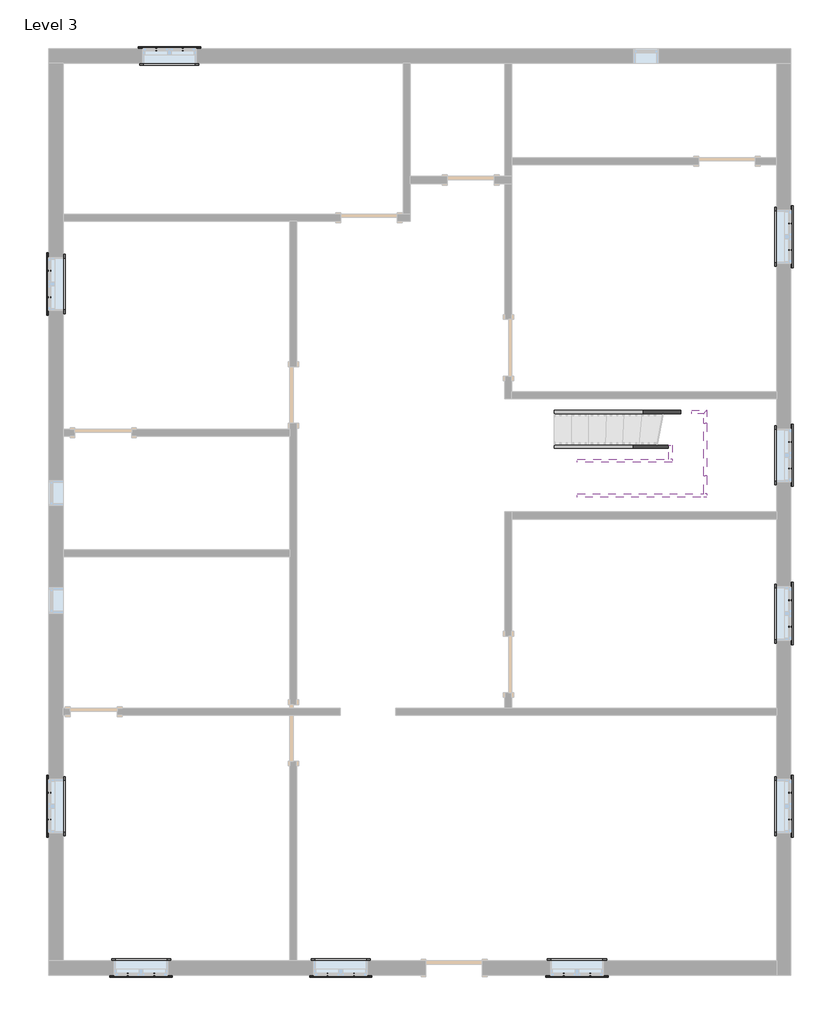
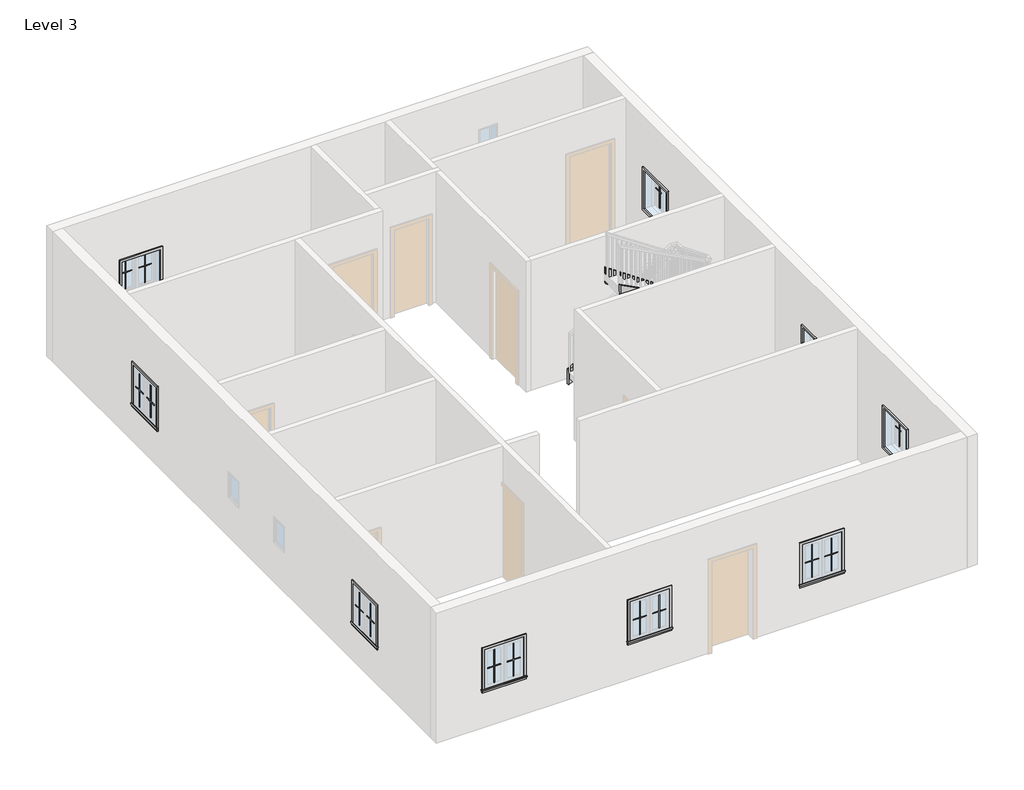
# One storey, part 3 of 3: 40 proxies, 9 members.
"""IFC4 building model written with IfcOpenShell, lengths in millimetres."""

from ifc_helpers import new_model, si_unit, frame, origin, place, context, project, spatial, polyline, outline, extrude, transform, mapped, element, save
from components import muntin_pattern_2x2_muntin_pattern_2x2_b3fe6957, muntin_pattern_2x2_muntin_pattern_2x2_3e0ecaf2, trim_window_exterior_flat_with_sill_41619996, trim_window_interior_flat_picture_frame_51c85655

model = new_model("IFC4")

# Units and contexts
model_context = context("Model", 3, world=origin())
ifc_project = project(units=[si_unit("LENGTHUNIT", "METRE", prefix="MILLI")], contexts=[model_context])

# Site, building, storey
site = spatial("IfcSite", under=ifc_project)
building = spatial("IfcBuilding", under=site)
storey = spatial("IfcBuildingStorey", under=building, Name="Level 3", Elevation=3200.4)

# Proxies
placement = place(None, origin())
muntin_pattern_2x2_muntin_pattern_2x2_shape = muntin_pattern_2x2_muntin_pattern_2x2_b3fe6957(model_context)
element("IfcBuildingElementProxy", 1, Name="Muntin Pattern_2x2 : Muntin Pattern_2x2", ObjectType="Muntin Pattern_2x2 : Muntin Pattern_2x2", at=placement, inside=storey, context=model_context, shape_type="MappedRepresentation", body=[
    mapped(muntin_pattern_2x2_muntin_pattern_2x2_shape, transform((-5581.2368007, 9072.452558, 4184.65), x_axis=(1.0, 0.0, 0.0), y_axis=(0.0, 1.0, 0.0), z_axis=(0.0, 0.0, 1.0))),
])
element("IfcBuildingElementProxy", 2, Name="Muntin Pattern_2x2 : Muntin Pattern_2x2", ObjectType="Muntin Pattern_2x2 : Muntin Pattern_2x2", at=placement, inside=storey, context=model_context, shape_type="MappedRepresentation", body=[
    mapped(muntin_pattern_2x2_muntin_pattern_2x2_shape, transform((-7300.4993007, 5076.715058, 4184.65), x_axis=(0.0, 1.0, 0.0), y_axis=(-1.0, 0.0, 0.0), z_axis=(0.0, 0.0, 1.0))),
])
element("IfcBuildingElementProxy", 3, Name="Muntin Pattern_2x2 : Muntin Pattern_2x2", ObjectType="Muntin Pattern_2x2 : Muntin Pattern_2x2", at=placement, inside=storey, context=model_context, shape_type="MappedRepresentation", body=[
    mapped(muntin_pattern_2x2_muntin_pattern_2x2_shape, transform((4643.8506993, 6267.340058, 4184.65), x_axis=(0.0, -1.0, 0.0), y_axis=(1.0, 0.0, 0.0), z_axis=(0.0, 0.0, 1.0))),
])
element("IfcBuildingElementProxy", 4, Name="Muntin Pattern_2x2 : Muntin Pattern_2x2", ObjectType="Muntin Pattern_2x2 : Muntin Pattern_2x2", at=placement, inside=storey, context=model_context, shape_type="MappedRepresentation", body=[
    mapped(muntin_pattern_2x2_muntin_pattern_2x2_shape, transform((4643.8506993, 2743.090058, 4184.65), x_axis=(0.0, -1.0, 0.0), y_axis=(1.0, 0.0, 0.0), z_axis=(0.0, 0.0, 1.0))),
])
element("IfcBuildingElementProxy", 5, Name="Muntin Pattern_2x2 : Muntin Pattern_2x2", ObjectType="Muntin Pattern_2x2 : Muntin Pattern_2x2", at=placement, inside=storey, context=model_context, shape_type="MappedRepresentation", body=[
    mapped(muntin_pattern_2x2_muntin_pattern_2x2_shape, transform((4643.8506993, 190.390058, 4184.65), x_axis=(0.0, -1.0, 0.0), y_axis=(1.0, 0.0, 0.0), z_axis=(0.0, 0.0, 1.0))),
])
element("IfcBuildingElementProxy", 6, Name="Muntin Pattern_2x2 : Muntin Pattern_2x2", ObjectType="Muntin Pattern_2x2 : Muntin Pattern_2x2", at=placement, inside=storey, context=model_context, shape_type="MappedRepresentation", body=[
    mapped(muntin_pattern_2x2_muntin_pattern_2x2_shape, transform((4643.8506993, -2914.759942, 4184.65), x_axis=(0.0, -1.0, 0.0), y_axis=(1.0, 0.0, 0.0), z_axis=(0.0, 0.0, 1.0))),
])
element("IfcBuildingElementProxy", 7, Name="Muntin Pattern_2x2 : Muntin Pattern_2x2", ObjectType="Muntin Pattern_2x2 : Muntin Pattern_2x2", at=placement, inside=storey, context=model_context, shape_type="MappedRepresentation", body=[
    mapped(muntin_pattern_2x2_muntin_pattern_2x2_shape, transform((1419.6381993, -5843.697442, 4184.65), x_axis=(-1.0, 0.0, 0.0), y_axis=(0.0, -1.0, 0.0), z_axis=(0.0, 0.0, 1.0))),
])
element("IfcBuildingElementProxy", 8, Name="Muntin Pattern_2x2 : Muntin Pattern_2x2", ObjectType="Muntin Pattern_2x2 : Muntin Pattern_2x2", at=placement, inside=storey, context=model_context, shape_type="MappedRepresentation", body=[
    mapped(muntin_pattern_2x2_muntin_pattern_2x2_shape, transform((-2390.3618007, -5843.697442, 4184.65), x_axis=(-1.0, 0.0, 0.0), y_axis=(0.0, -1.0, 0.0), z_axis=(0.0, 0.0, 1.0))),
])
element("IfcBuildingElementProxy", 9, Name="Muntin Pattern_2x2 : Muntin Pattern_2x2", ObjectType="Muntin Pattern_2x2 : Muntin Pattern_2x2", at=placement, inside=storey, context=model_context, shape_type="MappedRepresentation", body=[
    mapped(muntin_pattern_2x2_muntin_pattern_2x2_shape, transform((-5609.8118007, -5843.697442, 4184.65), x_axis=(-1.0, 0.0, 0.0), y_axis=(0.0, -1.0, 0.0), z_axis=(0.0, 0.0, 1.0))),
])
element("IfcBuildingElementProxy", 10, Name="Muntin Pattern_2x2 : Muntin Pattern_2x2", ObjectType="Muntin Pattern_2x2 : Muntin Pattern_2x2", at=placement, inside=storey, context=model_context, shape_type="MappedRepresentation", body=[
    mapped(muntin_pattern_2x2_muntin_pattern_2x2_shape, transform((-7300.4993007, -3343.384942, 4184.65), x_axis=(0.0, 1.0, 0.0), y_axis=(-1.0, 0.0, 0.0), z_axis=(0.0, 0.0, 1.0))),
])
muntin_pattern_2x2_muntin_pattern_2x2_2_shape = muntin_pattern_2x2_muntin_pattern_2x2_3e0ecaf2(model_context)
element("IfcBuildingElementProxy", 11, Name="Muntin Pattern_2x2 : Muntin Pattern_2x2", ObjectType="Muntin Pattern_2x2 : Muntin Pattern_2x2", at=placement, inside=storey, context=model_context, shape_type="MappedRepresentation", body=[
    mapped(muntin_pattern_2x2_muntin_pattern_2x2_2_shape, transform((-5152.6118007, 9072.452558, 4184.65), x_axis=(-1.0, 0.0, 0.0), y_axis=(0.0, -1.0, 0.0), z_axis=(0.0, 0.0, 1.0))),
])
element("IfcBuildingElementProxy", 12, Name="Muntin Pattern_2x2 : Muntin Pattern_2x2", ObjectType="Muntin Pattern_2x2 : Muntin Pattern_2x2", at=placement, inside=storey, context=model_context, shape_type="MappedRepresentation", body=[
    mapped(muntin_pattern_2x2_muntin_pattern_2x2_2_shape, transform((-7300.4993007, 5505.340058, 4184.65), x_axis=(0.0, -1.0, 0.0), y_axis=(1.0, 0.0, 0.0), z_axis=(0.0, 0.0, 1.0))),
])
element("IfcBuildingElementProxy", 13, Name="Muntin Pattern_2x2 : Muntin Pattern_2x2", ObjectType="Muntin Pattern_2x2 : Muntin Pattern_2x2", at=placement, inside=storey, context=model_context, shape_type="MappedRepresentation", body=[
    mapped(muntin_pattern_2x2_muntin_pattern_2x2_2_shape, transform((4643.8506993, 5838.715058, 4184.65), x_axis=(0.0, 1.0, 0.0), y_axis=(-1.0, 0.0, 0.0), z_axis=(0.0, 0.0, 1.0))),
])
element("IfcBuildingElementProxy", 14, Name="Muntin Pattern_2x2 : Muntin Pattern_2x2", ObjectType="Muntin Pattern_2x2 : Muntin Pattern_2x2", at=placement, inside=storey, context=model_context, shape_type="MappedRepresentation", body=[
    mapped(muntin_pattern_2x2_muntin_pattern_2x2_2_shape, transform((4643.8506993, 2314.465058, 4184.65), x_axis=(0.0, 1.0, 0.0), y_axis=(-1.0, 0.0, 0.0), z_axis=(0.0, 0.0, 1.0))),
])
element("IfcBuildingElementProxy", 15, Name="Muntin Pattern_2x2 : Muntin Pattern_2x2", ObjectType="Muntin Pattern_2x2 : Muntin Pattern_2x2", at=placement, inside=storey, context=model_context, shape_type="MappedRepresentation", body=[
    mapped(muntin_pattern_2x2_muntin_pattern_2x2_2_shape, transform((4643.8506993, -238.234942, 4184.65), x_axis=(0.0, 1.0, 0.0), y_axis=(-1.0, 0.0, 0.0), z_axis=(0.0, 0.0, 1.0))),
])
element("IfcBuildingElementProxy", 16, Name="Muntin Pattern_2x2 : Muntin Pattern_2x2", ObjectType="Muntin Pattern_2x2 : Muntin Pattern_2x2", at=placement, inside=storey, context=model_context, shape_type="MappedRepresentation", body=[
    mapped(muntin_pattern_2x2_muntin_pattern_2x2_2_shape, transform((4643.8506993, -3343.384942, 4184.65), x_axis=(0.0, 1.0, 0.0), y_axis=(-1.0, 0.0, 0.0), z_axis=(0.0, 0.0, 1.0))),
])
element("IfcBuildingElementProxy", 17, Name="Muntin Pattern_2x2 : Muntin Pattern_2x2", ObjectType="Muntin Pattern_2x2 : Muntin Pattern_2x2", at=placement, inside=storey, context=model_context, shape_type="MappedRepresentation", body=[
    mapped(muntin_pattern_2x2_muntin_pattern_2x2_2_shape, transform((991.0131993, -5843.697442, 4184.65), x_axis=(1.0, 0.0, 0.0), y_axis=(0.0, 1.0, 0.0), z_axis=(0.0, 0.0, 1.0))),
])
element("IfcBuildingElementProxy", 18, Name="Muntin Pattern_2x2 : Muntin Pattern_2x2", ObjectType="Muntin Pattern_2x2 : Muntin Pattern_2x2", at=placement, inside=storey, context=model_context, shape_type="MappedRepresentation", body=[
    mapped(muntin_pattern_2x2_muntin_pattern_2x2_2_shape, transform((-2818.9868007, -5843.697442, 4184.65), x_axis=(1.0, 0.0, 0.0), y_axis=(0.0, 1.0, 0.0), z_axis=(0.0, 0.0, 1.0))),
])
element("IfcBuildingElementProxy", 19, Name="Muntin Pattern_2x2 : Muntin Pattern_2x2", ObjectType="Muntin Pattern_2x2 : Muntin Pattern_2x2", at=placement, inside=storey, context=model_context, shape_type="MappedRepresentation", body=[
    mapped(muntin_pattern_2x2_muntin_pattern_2x2_2_shape, transform((-6038.4368007, -5843.697442, 4184.65), x_axis=(1.0, 0.0, 0.0), y_axis=(0.0, 1.0, 0.0), z_axis=(0.0, 0.0, 1.0))),
])
element("IfcBuildingElementProxy", 20, Name="Muntin Pattern_2x2 : Muntin Pattern_2x2", ObjectType="Muntin Pattern_2x2 : Muntin Pattern_2x2", at=placement, inside=storey, context=model_context, shape_type="MappedRepresentation", body=[
    mapped(muntin_pattern_2x2_muntin_pattern_2x2_2_shape, transform((-7300.4993007, -2914.759942, 4184.65), x_axis=(0.0, -1.0, 0.0), y_axis=(1.0, 0.0, 0.0), z_axis=(0.0, 0.0, 1.0))),
])
trim_window_exterior_flat_with_sill_shape = trim_window_exterior_flat_with_sill_41619996(model_context)
element("IfcBuildingElementProxy", 21, Name="Trim-Window-Exterior-Flat : with Sill", ObjectType="Trim-Window-Exterior-Flat : with Sill", at=placement, inside=storey, context=model_context, shape_type="MappedRepresentation", body=[
    mapped(trim_window_exterior_flat_with_sill_shape, transform((-5366.9243007, 9081.977558, 5029.2), x_axis=(-1.0, 0.0, 0.0), y_axis=(0.0, 0.0, 1.0), z_axis=(0.0, 1.0, 0.0))),
])
element("IfcBuildingElementProxy", 22, Name="Trim-Window-Exterior-Flat : with Sill", ObjectType="Trim-Window-Exterior-Flat : with Sill", at=placement, inside=storey, context=model_context, shape_type="MappedRepresentation", body=[
    mapped(trim_window_exterior_flat_with_sill_shape, transform((-7310.0243007, 5291.027558, 5029.2), x_axis=(0.0, -1.0, 0.0), y_axis=(0.0, 0.0, 1.0), z_axis=(-1.0, 0.0, 0.0))),
])
element("IfcBuildingElementProxy", 23, Name="Trim-Window-Exterior-Flat : with Sill", ObjectType="Trim-Window-Exterior-Flat : with Sill", at=placement, inside=storey, context=model_context, shape_type="MappedRepresentation", body=[
    mapped(trim_window_exterior_flat_with_sill_shape, transform((4653.3756993, 6053.027558, 5029.2), x_axis=(0.0, 1.0, 0.0), y_axis=(0.0, 0.0, 1.0), z_axis=(1.0, 0.0, 0.0))),
])
element("IfcBuildingElementProxy", 24, Name="Trim-Window-Exterior-Flat : with Sill", ObjectType="Trim-Window-Exterior-Flat : with Sill", at=placement, inside=storey, context=model_context, shape_type="MappedRepresentation", body=[
    mapped(trim_window_exterior_flat_with_sill_shape, transform((4653.3756993, 2528.777558, 5029.2), x_axis=(0.0, 1.0, 0.0), y_axis=(0.0, 0.0, 1.0), z_axis=(1.0, 0.0, 0.0))),
])
element("IfcBuildingElementProxy", 25, Name="Trim-Window-Exterior-Flat : with Sill", ObjectType="Trim-Window-Exterior-Flat : with Sill", at=placement, inside=storey, context=model_context, shape_type="MappedRepresentation", body=[
    mapped(trim_window_exterior_flat_with_sill_shape, transform((4653.3756993, -23.922442, 5029.2), x_axis=(0.0, 1.0, 0.0), y_axis=(0.0, 0.0, 1.0), z_axis=(1.0, 0.0, 0.0))),
])
element("IfcBuildingElementProxy", 26, Name="Trim-Window-Exterior-Flat : with Sill", ObjectType="Trim-Window-Exterior-Flat : with Sill", at=placement, inside=storey, context=model_context, shape_type="MappedRepresentation", body=[
    mapped(trim_window_exterior_flat_with_sill_shape, transform((4653.3756993, -3129.072442, 5029.2), x_axis=(0.0, 1.0, 0.0), y_axis=(0.0, 0.0, 1.0), z_axis=(1.0, 0.0, 0.0))),
])
element("IfcBuildingElementProxy", 27, Name="Trim-Window-Exterior-Flat : with Sill", ObjectType="Trim-Window-Exterior-Flat : with Sill", at=placement, inside=storey, context=model_context, shape_type="MappedRepresentation", body=[
    mapped(trim_window_exterior_flat_with_sill_shape, transform((1205.3256993, -5853.222442, 5029.2), x_axis=(1.0, 0.0, 0.0), y_axis=(0.0, 0.0, 1.0), z_axis=(0.0, -1.0, 0.0))),
])
element("IfcBuildingElementProxy", 28, Name="Trim-Window-Exterior-Flat : with Sill", ObjectType="Trim-Window-Exterior-Flat : with Sill", at=placement, inside=storey, context=model_context, shape_type="MappedRepresentation", body=[
    mapped(trim_window_exterior_flat_with_sill_shape, transform((-2604.6743007, -5853.222442, 5029.2), x_axis=(1.0, 0.0, 0.0), y_axis=(0.0, 0.0, 1.0), z_axis=(0.0, -1.0, 0.0))),
])
element("IfcBuildingElementProxy", 29, Name="Trim-Window-Exterior-Flat : with Sill", ObjectType="Trim-Window-Exterior-Flat : with Sill", at=placement, inside=storey, context=model_context, shape_type="MappedRepresentation", body=[
    mapped(trim_window_exterior_flat_with_sill_shape, transform((-5824.1243007, -5853.222442, 5029.2), x_axis=(1.0, 0.0, 0.0), y_axis=(0.0, 0.0, 1.0), z_axis=(0.0, -1.0, 0.0))),
])
element("IfcBuildingElementProxy", 30, Name="Trim-Window-Exterior-Flat : with Sill", ObjectType="Trim-Window-Exterior-Flat : with Sill", at=placement, inside=storey, context=model_context, shape_type="MappedRepresentation", body=[
    mapped(trim_window_exterior_flat_with_sill_shape, transform((-7310.0243007, -3129.072442, 5029.2), x_axis=(0.0, -1.0, 0.0), y_axis=(0.0, 0.0, 1.0), z_axis=(-1.0, 0.0, 0.0))),
])
trim_window_interior_flat_picture_frame_shape = trim_window_interior_flat_picture_frame_51c85655(model_context)
element("IfcBuildingElementProxy", 31, Name="Trim-Window-Interior-Flat : Picture Frame", ObjectType="Trim-Window-Interior-Flat : Picture Frame", at=placement, inside=storey, context=model_context, shape_type="MappedRepresentation", body=[
    mapped(trim_window_interior_flat_picture_frame_shape, transform((-5366.9243007, 8853.377558, 5029.2), x_axis=(1.0, 0.0, 0.0), y_axis=(0.0, 0.0, 1.0), z_axis=(0.0, -1.0, 0.0))),
])
element("IfcBuildingElementProxy", 32, Name="Trim-Window-Interior-Flat : Picture Frame", ObjectType="Trim-Window-Interior-Flat : Picture Frame", at=placement, inside=storey, context=model_context, shape_type="MappedRepresentation", body=[
    mapped(trim_window_interior_flat_picture_frame_shape, transform((-7081.4243007, 5291.027558, 5029.2), x_axis=(0.0, 1.0, 0.0), y_axis=(0.0, 0.0, 1.0), z_axis=(1.0, 0.0, 0.0))),
])
element("IfcBuildingElementProxy", 33, Name="Trim-Window-Interior-Flat : Picture Frame", ObjectType="Trim-Window-Interior-Flat : Picture Frame", at=placement, inside=storey, context=model_context, shape_type="MappedRepresentation", body=[
    mapped(trim_window_interior_flat_picture_frame_shape, transform((4424.7756993, 6053.027558, 5029.2), x_axis=(0.0, -1.0, 0.0), y_axis=(0.0, 0.0, 1.0), z_axis=(-1.0, 0.0, 0.0))),
])
element("IfcBuildingElementProxy", 34, Name="Trim-Window-Interior-Flat : Picture Frame", ObjectType="Trim-Window-Interior-Flat : Picture Frame", at=placement, inside=storey, context=model_context, shape_type="MappedRepresentation", body=[
    mapped(trim_window_interior_flat_picture_frame_shape, transform((4424.7756993, 2528.777558, 5029.2), x_axis=(0.0, -1.0, 0.0), y_axis=(0.0, 0.0, 1.0), z_axis=(-1.0, 0.0, 0.0))),
])
element("IfcBuildingElementProxy", 35, Name="Trim-Window-Interior-Flat : Picture Frame", ObjectType="Trim-Window-Interior-Flat : Picture Frame", at=placement, inside=storey, context=model_context, shape_type="MappedRepresentation", body=[
    mapped(trim_window_interior_flat_picture_frame_shape, transform((4424.7756993, -23.922442, 5029.2), x_axis=(0.0, -1.0, 0.0), y_axis=(0.0, 0.0, 1.0), z_axis=(-1.0, 0.0, 0.0))),
])
element("IfcBuildingElementProxy", 36, Name="Trim-Window-Interior-Flat : Picture Frame", ObjectType="Trim-Window-Interior-Flat : Picture Frame", at=placement, inside=storey, context=model_context, shape_type="MappedRepresentation", body=[
    mapped(trim_window_interior_flat_picture_frame_shape, transform((4424.7756993, -3129.072442, 5029.2), x_axis=(0.0, -1.0, 0.0), y_axis=(0.0, 0.0, 1.0), z_axis=(-1.0, 0.0, 0.0))),
])
element("IfcBuildingElementProxy", 37, Name="Trim-Window-Interior-Flat : Picture Frame", ObjectType="Trim-Window-Interior-Flat : Picture Frame", at=placement, inside=storey, context=model_context, shape_type="MappedRepresentation", body=[
    mapped(trim_window_interior_flat_picture_frame_shape, transform((1205.3256993, -5624.622442, 5029.2), x_axis=(-1.0, 0.0, 0.0), y_axis=(0.0, 0.0, 1.0), z_axis=(0.0, 1.0, 0.0))),
])
element("IfcBuildingElementProxy", 38, Name="Trim-Window-Interior-Flat : Picture Frame", ObjectType="Trim-Window-Interior-Flat : Picture Frame", at=placement, inside=storey, context=model_context, shape_type="MappedRepresentation", body=[
    mapped(trim_window_interior_flat_picture_frame_shape, transform((-2604.6743007, -5624.622442, 5029.2), x_axis=(-1.0, 0.0, 0.0), y_axis=(0.0, 0.0, 1.0), z_axis=(0.0, 1.0, 0.0))),
])
element("IfcBuildingElementProxy", 39, Name="Trim-Window-Interior-Flat : Picture Frame", ObjectType="Trim-Window-Interior-Flat : Picture Frame", at=placement, inside=storey, context=model_context, shape_type="MappedRepresentation", body=[
    mapped(trim_window_interior_flat_picture_frame_shape, transform((-5824.1243007, -5624.622442, 5029.2), x_axis=(-1.0, 0.0, 0.0), y_axis=(0.0, 0.0, 1.0), z_axis=(0.0, 1.0, 0.0))),
])
element("IfcBuildingElementProxy", 40, Name="Trim-Window-Interior-Flat : Picture Frame", ObjectType="Trim-Window-Interior-Flat : Picture Frame", at=placement, inside=storey, context=model_context, shape_type="MappedRepresentation", body=[
    mapped(trim_window_interior_flat_picture_frame_shape, transform((-7081.4243007, -3129.072442, 5029.2), x_axis=(0.0, 1.0, 0.0), y_axis=(0.0, 0.0, 1.0), z_axis=(1.0, 0.0, 0.0))),
])

# Members
element("IfcMember", 41, ObjectType="Stringer - 2\" Width", at=placement, inside=storey, context=model_context, shape_type="SweptSolid", body=[
    extrude(outline(polyline([(3588.8746569, 838.4202681), (3238.2072902, 838.4202681), (4497.8160324, 3052.6525996), (4848.4833991, 3052.6525996), (3588.8746569, 838.4202681)])), frame((0.0, 3202.4524989, 0.0), z_axis=(0.0, 1.0, 0.0), x_axis=(0.0, 0.0, 1.0)), (0.0, 0.0, 1.0), 50.8),
])
element("IfcMember", 42, ObjectType="Stringer - 2\" Width", at=placement, inside=storey, context=model_context, shape_type="SweptSolid", body=[
    extrude(outline(polyline([(3052.6525996, 3202.4524989), (3052.6525996, 3253.2524989), (3298.782332, 3253.2524989), (3247.982332, 3202.4524989), (3052.6525996, 3202.4524989)])), frame((0.0, 0.0, 4497.8160324), z_axis=(0.0, 0.0, 1.0), x_axis=(1.0, 0.0, 0.0)), (0.0, 0.0, 1.0), 350.6673667),
])
element("IfcMember", 43, ObjectType="Stringer - 2\" Width", at=placement, inside=storey, context=model_context, shape_type="SweptSolid", body=[
    extrude(outline(polyline([(3247.982332, 3202.4524989), (3298.782332, 3253.2524989), (3298.782332, 3048.1586437), (3247.982332, 3048.1586437), (3247.982332, 3202.4524989)])), frame((0.0, 0.0, 4497.8160324), z_axis=(0.0, 0.0, 1.0), x_axis=(1.0, 0.0, 0.0)), (0.0, 0.0, 1.0), 350.6673667),
])
element("IfcMember", 44, ObjectType="Stringer - 2\" Width", at=placement, inside=storey, context=model_context, shape_type="SweptSolid", body=[
    extrude(outline(polyline([(3048.1586437, 4848.4833991), (3048.1586437, 4497.8160324), (2198.376501, 4853.3779505), (2198.376501, 5204.0453172), (3048.1586437, 4848.4833991)])), frame((3247.982332, 0.0, 0.0), z_axis=(1.0, 0.0, 0.0), x_axis=(0.0, 1.0, 0.0)), (0.0, 0.0, 1.0), 50.8),
])
element("IfcMember", 45, ObjectType="Stringer - 2\" Width", at=placement, inside=storey, context=model_context, shape_type="SweptSolid", body=[
    extrude(outline(polyline([(3247.982332, 2198.376501), (3298.782332, 2198.376501), (3298.782332, 1905.9026171), (3247.982332, 1905.9026171), (3247.982332, 2198.376501)])), frame((0.0, 0.0, 4862.3761112), z_axis=(0.0, 0.0, 1.0), x_axis=(1.0, 0.0, 0.0)), (0.0, 0.0, 1.0), 330.4053693),
])
element("IfcMember", 46, ObjectType="Stringer - 2\" Width", at=placement, inside=storey, context=model_context, shape_type="SweptSolid", body=[
    extrude(outline(polyline([(3574.4558321, 838.4202681), (3211.5163437, 838.4202681), (4407.5401496, 2688.6073911), (4770.4796379, 2688.6073911), (3574.4558321, 838.4202681)])), frame((0.0, 2643.077558, 0.0), z_axis=(0.0, 1.0, 0.0), x_axis=(0.0, 0.0, 1.0)), (0.0, 0.0, 1.0), 50.8),
])
element("IfcMember", 47, ObjectType="Stringer - 2\" Width", at=placement, inside=storey, context=model_context, shape_type="SweptSolid", body=[
    extrude(outline(polyline([(2693.877558, 4937.8149577), (2693.877558, 4490.5996268), (2465.277558, 4736.0439445), (2465.277558, 5183.2592754), (2693.877558, 4937.8149577)])), frame((2688.6073911, 0.0, 0.0), z_axis=(1.0, 0.0, 0.0), x_axis=(0.0, 1.0, 0.0)), (0.0, 0.0, 1.0), 50.8),
])
element("IfcMember", 48, ObjectType="Stringer - 2\" Width", at=placement, inside=storey, context=model_context, shape_type="SweptSolid", body=[
    extrude(outline(polyline([(4901.1150039, 2739.4073911), (5271.091358, 2739.4073911), (6322.2229383, 1211.6756993), (5952.2465842, 1211.6756993), (4901.1150039, 2739.4073911)])), frame((0.0, 2414.477558, 0.0), z_axis=(0.0, 1.0, 0.0), x_axis=(0.0, 0.0, 1.0)), (0.0, 0.0, 1.0), 50.8),
])
element("IfcMember", 49, ObjectType="Stringer - 2\" Width", at=placement, inside=storey, context=model_context, shape_type="SweptSolid", body=[
    extrude(outline(polyline([(4887.9814805, 3298.782332), (5166.3410006, 3298.782332), (6252.642202, 1211.6756993), (5922.2368327, 1211.6756993), (4887.9814805, 3198.7868271), (4887.9814805, 3298.782332)])), frame((0.0, 1855.1026171, 0.0), z_axis=(0.0, 1.0, 0.0), x_axis=(0.0, 0.0, 1.0)), (0.0, 0.0, 1.0), 50.8),
])

save(model, "model.ifc")

# Revit data of these elements
# Type "Muntin Pattern_2x2 : Muntin Pattern_2x2"
#   Width [instance default] = 4' - 0"
#   Thickness = 0' - 0 1/2"
#   Height [instance default] = 4' - 0"
#   Distance = 0' - 0 3/4"
#   Interior Material [instance default] = none
#   Exterior Material [instance default] = none
#   Default Elevation = 0
# Type "Trim-Window-Exterior-Flat : with Sill"
#   Trim Width = 0' - 2 1/4"
#   Trim Thickness_Picture Frame = 0' - 1 1/4"
#   Trim Thickness_with Sill = 0' - 0 3/4"
#   Sill Thickness = 0' - 1 1/4"
#   Opening Width [instance default] = 2' - 0"
#   Opening Height [instance default] = 3' - 0"
#   Default Elevation = 4' - 0"
#   Sill = yes
#   Picture Frame = no
#   Trim Material [instance default] = none
# Type "Trim-Window-Interior-Flat : Picture Frame"
#   Trim Thickness_Picture Frame = 0' - 1 1/4"
#   Trim Width = 0' - 2 1/4"
#   Trim Thickness_with Sill = 0' - 0 3/4"
#   Sill Thickness = 0' - 1 1/4"
#   Opening Width [instance default] = 2' - 0"
#   Opening Height [instance default] = 3' - 0"
#   Default Elevation = 4' - 0"
#   Sill = no
#   Picture Frame = yes
#   Trim Material [instance default] = none
# Elements 1, 2, 3, 4, 5, 6, 7, 8, 9, 10, 11, 12, 13, 14, 15, 16, 17, 18, 19, 20 (IfcBuildingElementProxy, "Muntin Pattern_2x2 : Muntin Pattern_2x2")
#   Width = 0' - 11 5/8"
#   Height = 2' - 6 1/2"
#   Interior Material = Wood - Stained
#   Exterior Material = Clad - White
#   Phase Created = New Construction
#   Materials on its faces: "Clad - White", "Wood - Stained"
# Elements 21, 22, 23, 24, 25, 26, 27, 28, 29, 30 (IfcBuildingElementProxy, "Trim-Window-Exterior-Flat : with Sill")
#   Opening Width = 2' - 10"
#   Opening Height = 3' - 0"
#   Trim Material = Clad - White
#   Phase Created = New Construction
#   Materials on its faces: "Clad - White"
# Elements 31, 32, 33, 34, 35, 36, 37, 38, 39, 40 (IfcBuildingElementProxy, "Trim-Window-Interior-Flat : Picture Frame")
#   Opening Width = 2' - 10"
#   Opening Height = 3' - 0"
#   Trim Material = Wood - Stained
#   Phase Created = New Construction
#   Materials on its faces: "Wood - Stained"
# Elements 41, 42, 43, 44, 45, 46, 47, 48, 49 (IfcMember, "Stringer - 2\" Width")
#   Phase Created = New Construction
# Materials
#   "Clad - White": class "Wood", colour RGB 242 242 238, transparency 0, Cost = 0
#   "Wood - Stained": class "Wood", colour RGB 224 178 126, transparency 0, Cost = 0
